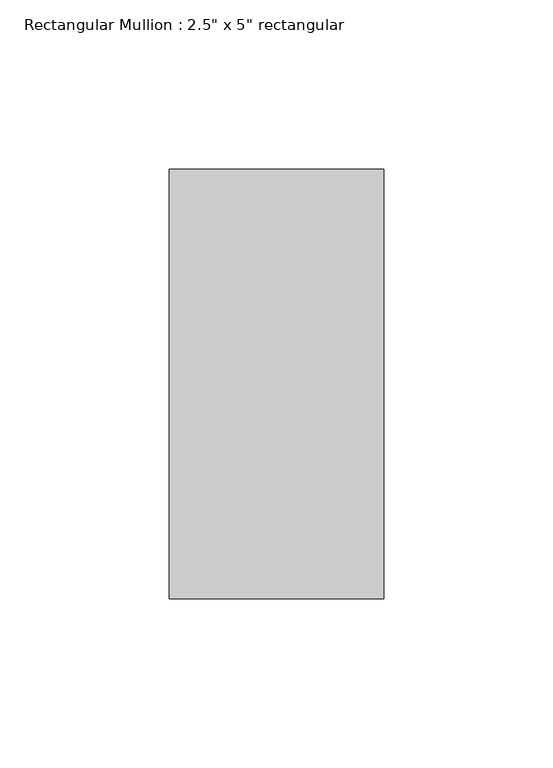
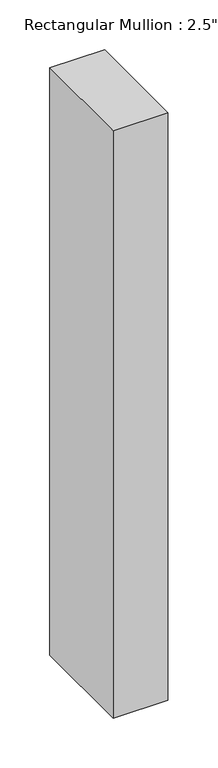
"""IFC4 building model written with IfcOpenShell, lengths in millimetres: member geometry."""

from ifc_helpers import new_model, si_unit, frame, origin, place, context, project, spatial, polyline, outline, extrude, source, transform, mapped, element, save


def member_09784a4a(model_context):
    return source(origin(), model_context, "Body", "SweptSolid", [
        extrude(outline(polyline([(0.0, 63.5), (0.0, -63.5), (-63.5, -63.5), (-63.5, 63.5), (0.0, 63.5)])), frame((0.0, 0.0, -719.8085391), z_axis=(0.0, 0.0, 1.0), x_axis=(1.0, 0.0, 0.0)), (0.0, 0.0, 1.0), 719.8085391),
    ])


if __name__ == "__main__":
    model = new_model("IFC4")
    model_context = context("Model", 3, world=origin())
    ifc_project = project(units=[si_unit("LENGTHUNIT", "METRE", prefix="MILLI")], contexts=[model_context])
    site = spatial("IfcSite", under=ifc_project)
    building = spatial("IfcBuilding", under=site)
    placement = place(None, origin())
    member_shape = member_09784a4a(model_context)
    element("IfcMember", 1, ObjectType="Rectangular Mullion : 2.5\" x 5\" rectangular", at=placement, inside=building, context=model_context, shape_type="MappedRepresentation", body=[
        mapped(member_shape, transform((0.0, 0.0, 0.0), x_axis=(1.0, 0.0, 0.0), y_axis=(0.0, 1.0, 0.0), z_axis=(0.0, 0.0, 1.0))),
    ])
    save(model, "model.ifc")

# Revit data of these elements
# Type "Rectangular Mullion : 2.5\" x 5\" rectangular"
#   built-in parameter 1007304 = 0.416667 (stored number, unit not read)
#   built-in parameter 1007301 = 0.104167 (stored number, unit not read)
#   built-in parameter 1007300 = 0.104167 (stored number, unit not read)
# Element 1 (IfcMember, "Rectangular Mullion : 2.5\" x 5\" rectangular")
#   Materials on its faces: "Aluminum"
# Materials
#   "Aluminum": class "Metal", colour RGB 247 247 247, transparency 0, Description = "Aluminum 6061", Cost = 0
